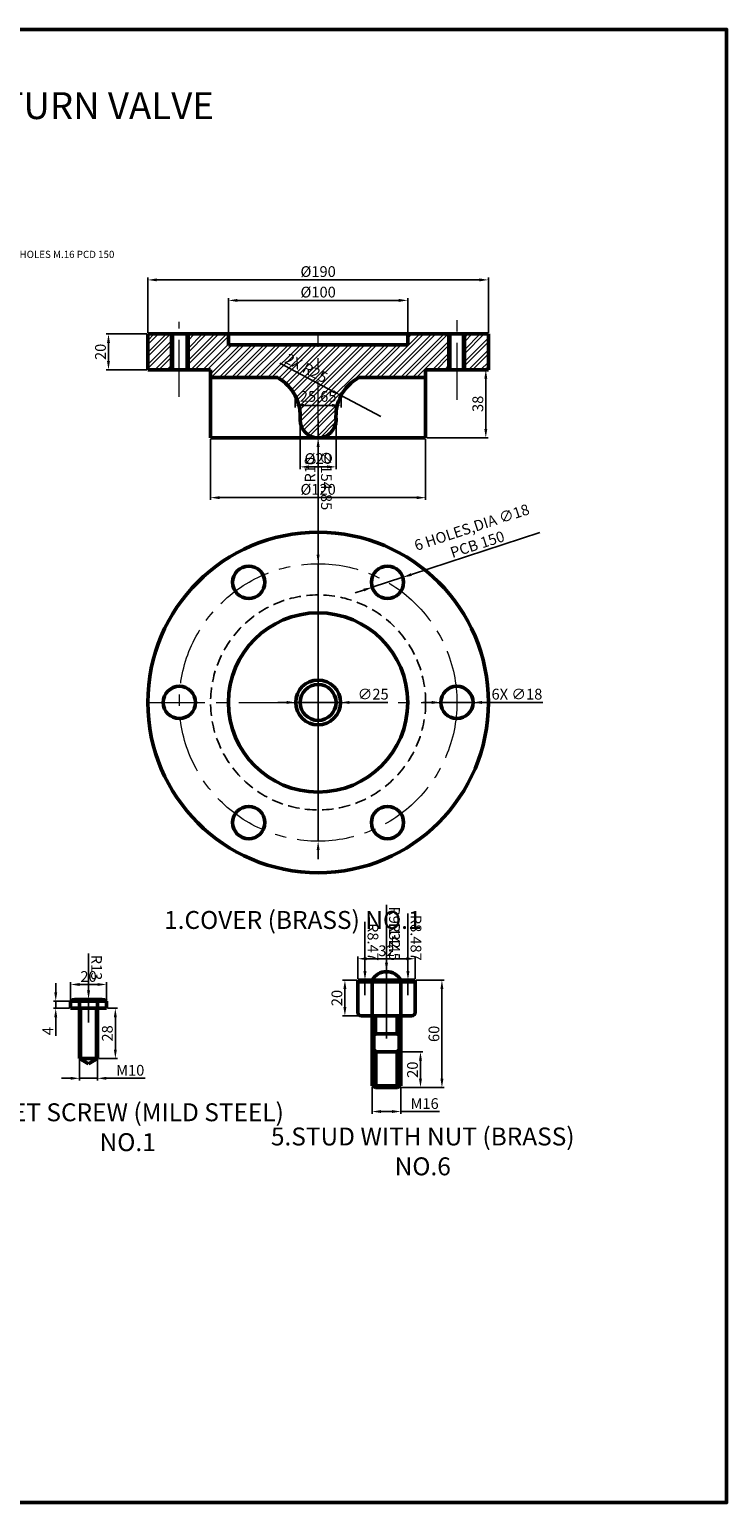
# Model space of a CAD drawing. Units: millimetres. Extents: x -907 to -46, y -312 to 510.
# Tile 3 of 3: x -434 to -46, y -312 to 510. Entities that reach past the tile are written whole.
import ezdxf
from ezdxf import colors
from ezdxf.entities.mleader import LeaderData, LeaderLine
from ezdxf.math import Vec2, Vec3

# ---------------------------------------------------------------- set-up
doc = ezdxf.new("R2010")
doc.units = ezdxf.units.MM
doc.linetypes.add('CENTER', pattern=[50.8, 31.75, -6.35, 6.35, -6.35])
doc.linetypes.add('HIDDEN', pattern=[9.525, 6.35, -3.175])
for name, color, linetype, lineweight in [('M-CNTR', 1, 'CENTER', 18), ('M-DIMS', 2, 'Continuous', 25), ('M-HATC', 8, 'Continuous', 18), ('M-HIDN', 6, 'HIDDEN', 25), ('M-OUTL', 7, 'Continuous', 50), ('M-TEXT', 3, 'Continuous', 25), ('M-TTLB', 7, 'Continuous', 50)]:
    doc.layers.add(name, color=color, linetype=linetype, lineweight=lineweight)
doc.styles.get("Standard").update_dxf_attribs({"font": 'arial.ttf'})
doc.dimstyles.new('ISO-25', dxfattribs={"dimtxt": 6, "dimasz": 5, "dimexe": 1.25, "dimexo": 0.625, "dimtad": 1, "dimtxsty": 'Standard', "dimcen": 2.5, "dimadec": 0, "dimazin": 0, "dimtfac": 1, "dimtmove": 0, "dimatfit": 3, "dimfxl": 1, "dimarcsym": 0})

# ---------------------------------------------------------------- blocks, each defined once
blk = doc.blocks.new('*D31')
at = {"layer": 'Defpoints', "color": 0, "transparency": 16777216}
for p in [(-178.39, 370.17), (-368.39, 340), (-178.39, 340)]:
    blk.add_point(p, dxfattribs=at)
at = {"layer": 'M-DIMS', "color": 0, "lineweight": -2, "transparency": 16777216}
for p, q in [((-368.39, 340.62), (-368.39, 371.42)), ((-363.39, 370.17), (-183.39, 370.17)), ((-178.39, 340.62), (-178.39, 371.42))]:
    blk.add_line(p, q, dxfattribs=at)
at = {"layer": 'M-DIMS', "color": 0, "transparency": 16777216}
for points in [[(-363.39, 371.01), (-363.39, 369.34), (-368.39, 370.17)], [(-183.39, 371.01), (-183.39, 369.34), (-178.39, 370.17)]]:
    blk.add_solid(points, dxfattribs=at)
at = {"layer": 'M-DIMS', "color": 0, "transparency": 16777216, "insert": (-273.39, 374.03), "char_height": 6, "attachment_point": 5}
blk.add_mtext('%%C190', dxfattribs=at)
blk = doc.blocks.new('*D32')
at = {"layer": 'Defpoints', "color": 0, "transparency": 16777216}
for p in [(-223.39, 358.73), (-323.39, 340), (-223.39, 340)]:
    blk.add_point(p, dxfattribs=at)
at = {"layer": 'M-DIMS', "color": 0, "lineweight": -2, "transparency": 16777216}
for p, q in [((-323.39, 340.62), (-323.39, 359.98)), ((-318.39, 358.73), (-228.39, 358.73)), ((-223.39, 340.62), (-223.39, 359.98))]:
    blk.add_line(p, q, dxfattribs=at)
at = {"layer": 'M-DIMS', "color": 0, "transparency": 16777216}
for points in [[(-318.39, 359.56), (-318.39, 357.89), (-323.39, 358.73)], [(-228.39, 359.56), (-228.39, 357.89), (-223.39, 358.73)]]:
    blk.add_solid(points, dxfattribs=at)
at = {"layer": 'M-DIMS', "color": 0, "transparency": 16777216, "insert": (-273.39, 362.58), "char_height": 6, "attachment_point": 5}
blk.add_mtext('%%C100', dxfattribs=at)
blk = doc.blocks.new('*D33')
at = {"layer": 'Defpoints', "color": 0, "transparency": 16777216}
for p in [(-368.39, 340), (-390.36, 320), (-368.39, 320)]:
    blk.add_point(p, dxfattribs=at)
at = {"layer": 'M-DIMS', "color": 0, "lineweight": -2, "transparency": 16777216}
for p, q in [((-369.02, 340), (-391.61, 340)), ((-390.36, 335), (-390.36, 325)), ((-369.02, 320), (-391.61, 320))]:
    blk.add_line(p, q, dxfattribs=at)
at = {"layer": 'M-DIMS', "color": 0, "transparency": 16777216}
for points in [[(-391.19, 335), (-389.53, 335), (-390.36, 340)], [(-391.19, 325), (-389.53, 325), (-390.36, 320)]]:
    blk.add_solid(points, dxfattribs=at)
at = {"layer": 'M-DIMS', "color": 0, "transparency": 16777216, "insert": (-394.05, 330), "char_height": 6, "attachment_point": 5, "rotation": 90}
blk.add_mtext('20', dxfattribs=at)
blk = doc.blocks.new('*D34')
at = {"layer": 'Defpoints', "color": 0, "transparency": 16777216}
for p in [(-283.39, 292), (-263.39, 292), (-263.39, 265.83)]:
    blk.add_point(p, dxfattribs=at)
at = {"layer": 'M-DIMS', "color": 0, "lineweight": -2, "transparency": 16777216}
for p, q in [((-283.39, 291.37), (-283.39, 264.58)), ((-263.39, 291.37), (-263.39, 264.58)), ((-278.39, 265.83), (-268.39, 265.83))]:
    blk.add_line(p, q, dxfattribs=at)
at = {"layer": 'M-DIMS', "color": 0, "transparency": 16777216}
for points in [[(-278.39, 266.66), (-278.39, 265), (-283.39, 265.83)], [(-268.39, 266.66), (-268.39, 265), (-263.39, 265.83)]]:
    blk.add_solid(points, dxfattribs=at)
at = {"layer": 'M-DIMS', "color": 0, "transparency": 16777216, "insert": (-273.39, 269.69), "char_height": 6, "attachment_point": 5}
blk.add_mtext('%%C20', dxfattribs=at)
blk = doc.blocks.new('*D35')
at = {"layer": 'Defpoints', "color": 0, "transparency": 16777216}
for p in [(-333.39, 282), (-213.39, 282), (-213.39, 248.65)]:
    blk.add_point(p, dxfattribs=at)
at = {"layer": 'M-DIMS', "color": 0, "lineweight": -2, "transparency": 16777216}
for p, q in [((-333.39, 281.37), (-333.39, 247.4)), ((-213.39, 281.37), (-213.39, 247.4)), ((-328.39, 248.65), (-218.39, 248.65))]:
    blk.add_line(p, q, dxfattribs=at)
at = {"layer": 'M-DIMS', "color": 0, "transparency": 16777216}
for points in [[(-328.39, 249.48), (-328.39, 247.82), (-333.39, 248.65)], [(-218.39, 249.48), (-218.39, 247.82), (-213.39, 248.65)]]:
    blk.add_solid(points, dxfattribs=at)
at = {"layer": 'M-DIMS', "color": 0, "transparency": 16777216, "insert": (-273.39, 252.51), "char_height": 6, "attachment_point": 5}
blk.add_mtext('%%C120', dxfattribs=at)
blk = doc.blocks.new('*D36')
at = {"layer": 'Defpoints', "color": 0, "transparency": 16777216}
for p in [(-286.22, 305.62), (-260.57, 305.62), (-260.57, 300.14)]:
    blk.add_point(p, dxfattribs=at)
at = {"layer": 'M-DIMS', "color": 0, "lineweight": -2, "transparency": 16777216}
for p, q in [((-286.22, 305), (-286.22, 298.89)), ((-260.57, 305), (-260.57, 298.89)), ((-281.22, 300.14), (-265.57, 300.14))]:
    blk.add_line(p, q, dxfattribs=at)
at = {"layer": 'M-DIMS', "color": 0, "transparency": 16777216}
for points in [[(-281.22, 300.97), (-281.22, 299.31), (-286.22, 300.14)], [(-265.57, 300.97), (-265.57, 299.31), (-260.57, 300.14)]]:
    blk.add_solid(points, dxfattribs=at)
at = {"layer": 'M-DIMS', "color": 0, "transparency": 16777216, "insert": (-273.39, 304.37), "char_height": 6, "attachment_point": 5}
blk.add_mtext('25,65', dxfattribs=at)
blk = doc.blocks.new('*D37')
at = {"layer": 'Defpoints', "color": 0, "transparency": 16777216}
for p in [(-213.39, 320), (-213.39, 282), (-179.83, 282)]:
    blk.add_point(p, dxfattribs=at)
at = {"layer": 'M-DIMS', "color": 0, "lineweight": -2, "transparency": 16777216}
for p, q in [((-212.77, 320), (-178.58, 320)), ((-179.83, 315), (-179.83, 287)), ((-212.77, 282), (-178.58, 282))]:
    blk.add_line(p, q, dxfattribs=at)
at = {"layer": 'M-DIMS', "color": 0, "transparency": 16777216}
for points in [[(-180.66, 315), (-179, 315), (-179.83, 320)], [(-180.66, 287), (-179, 287), (-179.83, 282)]]:
    blk.add_solid(points, dxfattribs=at)
at = {"layer": 'M-DIMS', "color": 0, "transparency": 16777216, "insert": (-183.52, 301), "char_height": 6, "attachment_point": 5, "rotation": 90}
blk.add_mtext('38', dxfattribs=at)
blk = doc.blocks.new('*D38')
at = {"layer": 'Defpoints', "color": 0, "transparency": 16777216}
for p in [(-243.24, 198.61), (-226.12, 204.19)]:
    blk.add_point(p, dxfattribs=at)
at = {"layer": 'M-DIMS', "color": 0, "lineweight": -2, "transparency": 16777216}
for p, q in [((-149.63, 229.11), (-221.37, 205.74)), ((-243.24, 198.61), (-226.12, 204.19)), ((-247.99, 197.07), (-252.75, 195.52))]:
    blk.add_line(p, q, dxfattribs=at)
at = {"layer": 'M-DIMS', "color": 0, "transparency": 16777216}
for points in [[(-221.63, 206.53), (-221.11, 204.95), (-226.12, 204.19)], [(-248.25, 197.86), (-247.73, 196.27), (-243.24, 198.61)]]:
    blk.add_solid(points, dxfattribs=at)
at = {"layer": 'M-DIMS', "color": 0, "transparency": 16777216, "insert": (-185.86, 226.6), "char_height": 6, "attachment_point": 5, "rotation": 18.0433}
blk.add_mtext('6 HOLES,DIA ∅18\\PPCB 150', dxfattribs=at)
blk = doc.blocks.new('*D49')
at = {"layer": 'Defpoints', "color": 0, "transparency": 16777216}
for p in [(-406.48, -64.34), (-396.48, -64.34), (-396.48, -75.39)]:
    blk.add_point(p, dxfattribs=at)
at = {"layer": 'M-DIMS', "color": 0, "lineweight": -2, "transparency": 16777216}
for p, q in [((-406.48, -64.97), (-406.48, -76.64)), ((-396.48, -64.97), (-396.48, -76.64)), ((-411.48, -75.39), (-416.48, -75.39)), ((-406.48, -75.39), (-396.48, -75.39)), ((-391.48, -75.39), (-369.95, -75.39))]:
    blk.add_line(p, q, dxfattribs=at)
at = {"layer": 'M-DIMS', "color": 0, "transparency": 16777216}
for points in [[(-411.48, -74.56), (-411.48, -76.23), (-406.48, -75.39)], [(-391.48, -74.56), (-391.48, -76.23), (-396.48, -75.39)]]:
    blk.add_solid(points, dxfattribs=at)
at = {"layer": 'M-DIMS', "color": 0, "transparency": 16777216, "insert": (-378.22, -71.7), "char_height": 6, "attachment_point": 5}
blk.add_mtext('M10', dxfattribs=at)
blk = doc.blocks.new('*D50')
at = {"layer": 'Defpoints', "color": 0, "transparency": 16777216}
for p in [(-219.25, -20.59), (-235.25, -80.59), (-204.32, -80.59)]:
    blk.add_point(p, dxfattribs=at)
at = {"layer": 'M-DIMS', "color": 0, "lineweight": -2, "transparency": 16777216}
for p, q in [((-218.63, -20.59), (-203.07, -20.59)), ((-204.32, -25.59), (-204.32, -75.59)), ((-234.63, -80.59), (-203.07, -80.59))]:
    blk.add_line(p, q, dxfattribs=at)
at = {"layer": 'M-DIMS', "color": 0, "transparency": 16777216}
for points in [[(-205.15, -25.59), (-203.48, -25.59), (-204.32, -20.59)], [(-205.15, -75.59), (-203.48, -75.59), (-204.32, -80.59)]]:
    blk.add_solid(points, dxfattribs=at)
at = {"layer": 'M-DIMS', "color": 0, "transparency": 16777216, "insert": (-208, -50.59), "char_height": 6, "attachment_point": 5, "rotation": 90}
blk.add_mtext('60', dxfattribs=at)
blk = doc.blocks.new('*D51')
at = {"layer": 'Defpoints', "color": 0, "transparency": 16777216}
for p in [(-235.25, -60.59), (-235.25, -80.59), (-216.29, -80.59)]:
    blk.add_point(p, dxfattribs=at)
at = {"layer": 'M-DIMS', "color": 0, "lineweight": -2, "transparency": 16777216}
for p, q in [((-234.63, -60.59), (-215.04, -60.59)), ((-216.29, -65.59), (-216.29, -75.59)), ((-234.63, -80.59), (-215.04, -80.59))]:
    blk.add_line(p, q, dxfattribs=at)
at = {"layer": 'M-DIMS', "color": 0, "transparency": 16777216}
for points in [[(-217.12, -65.59), (-215.45, -65.59), (-216.29, -60.59)], [(-217.12, -75.59), (-215.45, -75.59), (-216.29, -80.59)]]:
    blk.add_solid(points, dxfattribs=at)
at = {"layer": 'M-DIMS', "color": 0, "transparency": 16777216, "insert": (-219.97, -70.59), "char_height": 6, "attachment_point": 5, "rotation": 90}
blk.add_mtext('20', dxfattribs=at)
blk = doc.blocks.new('*D52')
at = {"layer": 'Defpoints', "color": 0, "transparency": 16777216}
for p in [(-243.25, -79.59), (-227.25, -79.59), (-227.25, -93.95)]:
    blk.add_point(p, dxfattribs=at)
at = {"layer": 'M-DIMS', "color": 0, "lineweight": -2, "transparency": 16777216}
for p, q in [((-243.25, -80.22), (-243.25, -95.2)), ((-227.25, -80.22), (-227.25, -95.2)), ((-238.25, -93.95), (-232.25, -93.95)), ((-227.25, -93.95), (-205.7, -93.95))]:
    blk.add_line(p, q, dxfattribs=at)
at = {"layer": 'M-DIMS', "color": 0, "transparency": 16777216}
for points in [[(-238.25, -93.11), (-238.25, -94.78), (-243.25, -93.95)], [(-232.25, -93.11), (-232.25, -94.78), (-227.25, -93.95)]]:
    blk.add_solid(points, dxfattribs=at)
at = {"layer": 'M-DIMS', "color": 0, "transparency": 16777216, "insert": (-213.98, -90.26), "char_height": 6, "attachment_point": 5}
blk.add_mtext('M16', dxfattribs=at)
blk = doc.blocks.new('*D53')
at = {"layer": 'Defpoints', "color": 0, "transparency": 16777216}
for p in [(-391.48, -36.34), (-396.48, -64.34), (-386.53, -64.34)]:
    blk.add_point(p, dxfattribs=at)
at = {"layer": 'M-DIMS', "color": 0, "lineweight": -2, "transparency": 16777216}
for p, q in [((-390.86, -36.34), (-385.28, -36.34)), ((-386.53, -41.34), (-386.53, -59.34)), ((-395.86, -64.34), (-385.28, -64.34))]:
    blk.add_line(p, q, dxfattribs=at)
at = {"layer": 'M-DIMS', "color": 0, "transparency": 16777216}
for points in [[(-387.36, -41.34), (-385.7, -41.34), (-386.53, -36.34)], [(-387.36, -59.34), (-385.7, -59.34), (-386.53, -64.34)]]:
    blk.add_solid(points, dxfattribs=at)
at = {"layer": 'M-DIMS', "color": 0, "transparency": 16777216, "insert": (-390.22, -50.34), "char_height": 6, "attachment_point": 5, "rotation": 90}
blk.add_mtext('28', dxfattribs=at)
blk = doc.blocks.new('HOLE-D18')
blk.add_circle((9, 9), 9)
blk = doc.blocks.new('*D57')
at = {"layer": 'Defpoints', "color": 0, "transparency": 16777216}
for p in [(-391.48, -23.04), (-411.48, -36.34), (-391.48, -36.34)]:
    blk.add_point(p, dxfattribs=at)
at = {"layer": 'M-DIMS', "color": 0, "lineweight": -2, "transparency": 16777216}
for p, q in [((-411.48, -35.72), (-411.48, -21.79)), ((-406.48, -23.04), (-396.48, -23.04)), ((-391.48, -35.72), (-391.48, -21.79))]:
    blk.add_line(p, q, dxfattribs=at)
at = {"layer": 'M-DIMS', "color": 0, "transparency": 16777216}
for points in [[(-406.48, -22.21), (-406.48, -23.87), (-411.48, -23.04)], [(-396.48, -22.21), (-396.48, -23.87), (-391.48, -23.04)]]:
    blk.add_solid(points, dxfattribs=at)
at = {"layer": 'M-DIMS', "color": 0, "transparency": 16777216, "insert": (-401.48, -19.35), "char_height": 6, "attachment_point": 5}
blk.add_mtext('20', dxfattribs=at)
blk = doc.blocks.new('*D58')
at = {"layer": 'Defpoints', "color": 0, "transparency": 16777216}
for p in [(-411.48, -32.34), (-419.78, -36.34), (-411.48, -36.34)]:
    blk.add_point(p, dxfattribs=at)
at = {"layer": 'M-DIMS', "color": 0, "lineweight": -2, "transparency": 16777216}
for p, q in [((-419.78, -27.34), (-419.78, -22.34)), ((-412.11, -32.34), (-421.03, -32.34)), ((-419.78, -32.34), (-419.78, -36.34)), ((-412.11, -36.34), (-421.03, -36.34)), ((-419.78, -41.34), (-419.78, -51.74))]:
    blk.add_line(p, q, dxfattribs=at)
at = {"layer": 'M-DIMS', "color": 0, "transparency": 16777216}
for points in [[(-420.62, -27.34), (-418.95, -27.34), (-419.78, -32.34)], [(-420.62, -41.34), (-418.95, -41.34), (-419.78, -36.34)]]:
    blk.add_solid(points, dxfattribs=at)
at = {"layer": 'M-DIMS', "color": 0, "transparency": 16777216, "insert": (-423.41, -49.04), "char_height": 6, "attachment_point": 5, "rotation": 90}
blk.add_mtext('4', dxfattribs=at)
blk = doc.blocks.new('*D59')
at = {"layer": 'Defpoints', "color": 0, "transparency": 16777216}
for p in [(-219.25, -8.68), (-251.25, -20.59), (-219.25, -20.59)]:
    blk.add_point(p, dxfattribs=at)
at = {"layer": 'M-DIMS', "color": 0, "lineweight": -2, "transparency": 16777216}
for p, q in [((-251.25, -19.97), (-251.25, -7.43)), ((-219.25, -19.97), (-219.25, -7.43)), ((-246.25, -8.68), (-224.25, -8.68))]:
    blk.add_line(p, q, dxfattribs=at)
at = {"layer": 'M-DIMS', "color": 0, "transparency": 16777216}
for points in [[(-246.25, -7.85), (-246.25, -9.51), (-251.25, -8.68)], [(-224.25, -7.85), (-224.25, -9.51), (-219.25, -8.68)]]:
    blk.add_solid(points, dxfattribs=at)
at = {"layer": 'M-DIMS', "color": 0, "transparency": 16777216, "insert": (-235.25, -4.99), "char_height": 6, "attachment_point": 5}
blk.add_mtext('32', dxfattribs=at)
blk = doc.blocks.new('*D60')
at = {"layer": 'Defpoints', "color": 0, "transparency": 16777216}
for p in [(-251.25, -20.59), (-258.45, -40.59), (-249.25, -40.59)]:
    blk.add_point(p, dxfattribs=at)
at = {"layer": 'M-DIMS', "color": 0, "lineweight": -2, "transparency": 16777216}
for p, q in [((-251.88, -20.59), (-259.7, -20.59)), ((-258.45, -25.59), (-258.45, -35.59)), ((-249.88, -40.59), (-259.7, -40.59))]:
    blk.add_line(p, q, dxfattribs=at)
at = {"layer": 'M-DIMS', "color": 0, "transparency": 16777216}
for points in [[(-259.29, -25.59), (-257.62, -25.59), (-258.45, -20.59)], [(-259.29, -35.59), (-257.62, -35.59), (-258.45, -40.59)]]:
    blk.add_solid(points, dxfattribs=at)
at = {"layer": 'M-DIMS', "color": 0, "transparency": 16777216, "insert": (-262.14, -30.59), "char_height": 6, "attachment_point": 5, "rotation": 90}
blk.add_mtext('20', dxfattribs=at)
blk = doc.blocks.new('*D64')
at = {"layer": 'Defpoints', "color": 0, "transparency": 16777216}
for p in [(-260.57, 305.62), (-238.47, 293.93)]:
    blk.add_point(p, dxfattribs=at)
at = {"layer": 'M-DIMS', "color": 0, "lineweight": -2, "transparency": 16777216}
for p, q in [((-294.71, 323.68), (-264.99, 307.96)), ((-238.47, 293.93), (-260.57, 305.62))]:
    blk.add_line(p, q, dxfattribs=at)
at = {"layer": 'M-DIMS', "color": 0, "transparency": 16777216}
blk.add_solid([(-264.6, 308.7), (-265.38, 307.22), (-260.57, 305.62)], dxfattribs=at)
at = {"layer": 'M-DIMS', "color": 0, "transparency": 16777216, "insert": (-280.33, 320.25), "char_height": 6, "attachment_point": 5, "rotation": 332.11935}
blk.add_mtext('2X R25', dxfattribs=at)
blk = doc.blocks.new('*D65')
at = {"layer": 'Defpoints', "color": 0, "transparency": 16777216}
for p in [(-273.39, 292), (-273.39, 282)]:
    blk.add_point(p, dxfattribs=at)
at = {"layer": 'M-DIMS', "color": 0, "lineweight": -2, "transparency": 16777216}
for p, q in [((-273.39, 292), (-273.39, 282)), ((-273.39, 256.43), (-273.39, 277))]:
    blk.add_line(p, q, dxfattribs=at)
at = {"layer": 'M-DIMS', "color": 0, "transparency": 16777216}
blk.add_solid([(-274.23, 277), (-272.56, 277), (-273.39, 282)], dxfattribs=at)
at = {"layer": 'M-DIMS', "color": 0, "transparency": 16777216, "insert": (-277.08, 264.21), "char_height": 6, "attachment_point": 5, "rotation": 89.99849}
blk.add_mtext('R10', dxfattribs=at)
blk = doc.blocks.new('*D66')
at = {"layer": 'Defpoints', "color": 0, "transparency": 16777216}
for p in [(-204.97, 134.35), (-186.97, 134.35)]:
    blk.add_point(p, dxfattribs=at)
at = {"layer": 'M-DIMS', "color": 0, "lineweight": -2, "transparency": 16777216}
for p, q in [((-209.97, 134.35), (-214.97, 134.35)), ((-204.97, 134.35), (-186.97, 134.35)), ((-147.98, 134.35), (-181.97, 134.35))]:
    blk.add_line(p, q, dxfattribs=at)
at = {"layer": 'M-DIMS', "color": 0, "transparency": 16777216}
for points in [[(-209.97, 135.19), (-209.97, 133.52), (-204.97, 134.35)], [(-181.97, 135.19), (-181.97, 133.52), (-186.97, 134.35)]]:
    blk.add_solid(points, dxfattribs=at)
at = {"layer": 'M-DIMS', "color": 0, "transparency": 16777216, "insert": (-162.47, 138.21), "char_height": 6, "attachment_point": 5, "rotation": 359.99799}
blk.add_mtext('6X ∅18', dxfattribs=at)
blk = doc.blocks.new('*D67')
at = {"layer": 'Defpoints', "color": 0, "transparency": 16777216}
for p in [(-273.39, 211.77), (-273.39, 56.93)]:
    blk.add_point(p, dxfattribs=at)
at = {"layer": 'M-DIMS', "color": 0, "lineweight": -2, "transparency": 16777216}
for p, q in [((-273.39, 274.59), (-273.39, 216.77)), ((-273.39, 56.93), (-273.39, 211.77)), ((-273.39, 51.93), (-273.39, 46.93))]:
    blk.add_line(p, q, dxfattribs=at)
at = {"layer": 'M-DIMS', "color": 0, "transparency": 16777216}
for points in [[(-272.56, 216.77), (-274.23, 216.77), (-273.39, 211.77)], [(-272.56, 51.93), (-274.23, 51.93), (-273.39, 56.93)]]:
    blk.add_solid(points, dxfattribs=at)
at = {"layer": 'M-DIMS', "color": 0, "transparency": 16777216, "insert": (-269.54, 258.23), "char_height": 6, "attachment_point": 5, "rotation": 270.00019}
blk.add_mtext('∅154.85', dxfattribs=at)
blk = doc.blocks.new('*D68')
at = {"layer": 'Defpoints', "color": 0, "transparency": 16777216}
for p in [(-285.89, 134.35), (-260.89, 134.35)]:
    blk.add_point(p, dxfattribs=at)
at = {"layer": 'M-DIMS', "color": 0, "lineweight": -2, "transparency": 16777216}
for p, q in [((-290.89, 134.35), (-295.89, 134.35)), ((-285.89, 134.35), (-260.89, 134.35)), ((-234.47, 134.35), (-255.89, 134.35))]:
    blk.add_line(p, q, dxfattribs=at)
at = {"layer": 'M-DIMS', "color": 0, "transparency": 16777216}
for points in [[(-290.89, 135.19), (-290.89, 133.52), (-285.89, 134.35)], [(-255.89, 135.19), (-255.89, 133.52), (-260.89, 134.35)]]:
    blk.add_solid(points, dxfattribs=at)
at = {"layer": 'M-DIMS', "color": 0, "transparency": 16777216, "insert": (-242.68, 138.21), "char_height": 6, "attachment_point": 5, "rotation": 359.99857}
blk.add_mtext('∅25', dxfattribs=at)
blk = doc.blocks.new('*D69')
at = {"layer": 'Defpoints', "color": 0, "transparency": 16777216}
for p in [(-401.48, -31.34), (-401.48, -44.34)]:
    blk.add_point(p, dxfattribs=at)
at = {"layer": 'M-DIMS', "color": 0, "lineweight": -2, "transparency": 16777216}
for p, q in [((-401.48, -5.75), (-401.48, -26.34)), ((-401.48, -44.34), (-401.48, -31.34))]:
    blk.add_line(p, q, dxfattribs=at)
at = {"layer": 'M-DIMS', "color": 0, "transparency": 16777216}
blk.add_solid([(-400.65, -26.34), (-402.32, -26.34), (-401.48, -31.34)], dxfattribs=at)
at = {"layer": 'M-DIMS', "color": 0, "transparency": 16777216, "insert": (-397.79, -13.55), "char_height": 6, "attachment_point": 5, "rotation": 270.00195}
blk.add_mtext('R13', dxfattribs=at)
blk = doc.blocks.new('*D70')
at = {"layer": 'Defpoints', "color": 0, "transparency": 16777216}
for p in [(-235.25, -20.59), (-235.25, -53.09)]:
    blk.add_point(p, dxfattribs=at)
at = {"layer": 'M-DIMS', "color": 0, "lineweight": -2, "transparency": 16777216}
for p, q in [((-235.25, 12.03), (-235.25, -15.59)), ((-235.25, -53.09), (-235.25, -20.59))]:
    blk.add_line(p, q, dxfattribs=at)
at = {"layer": 'M-DIMS', "color": 0, "transparency": 16777216}
blk.add_solid([(-234.42, -15.59), (-236.09, -15.59), (-235.25, -20.59)], dxfattribs=at)
at = {"layer": 'M-DIMS', "color": 0, "transparency": 16777216, "insert": (-231.56, 0.72), "char_height": 6, "attachment_point": 5, "rotation": 270.00062}
blk.add_mtext('R32.5', dxfattribs=at)
blk = doc.blocks.new('*D71')
at = {"layer": 'Defpoints', "color": 0, "transparency": 16777216}
for p in [(-235.25, -15.88), (-235.25, -25.02)]:
    blk.add_point(p, dxfattribs=at)
at = {"layer": 'M-DIMS', "color": 0, "lineweight": -2, "transparency": 16777216}
for p, q in [((-235.25, 21.34), (-235.25, -10.88)), ((-235.25, -25.02), (-235.25, -15.88))]:
    blk.add_line(p, q, dxfattribs=at)
at = {"layer": 'M-DIMS', "color": 0, "transparency": 16777216}
blk.add_solid([(-234.42, -10.88), (-236.09, -10.88), (-235.25, -15.88)], dxfattribs=at)
at = {"layer": 'M-DIMS', "color": 0, "transparency": 16777216, "insert": (-231.57, 7.73), "char_height": 6, "attachment_point": 5, "rotation": 270.0022}
blk.add_mtext('R9.144', dxfattribs=at)
blk = doc.blocks.new('*D72')
at = {"layer": 'Defpoints', "color": 0, "transparency": 16777216}
for p in [(-247.25, -20.59), (-247.25, -29.06)]:
    blk.add_point(p, dxfattribs=at)
at = {"layer": 'M-DIMS', "color": 0, "lineweight": -2, "transparency": 16777216}
for p, q in [((-247.25, 11.99), (-247.25, -15.59)), ((-247.25, -29.06), (-247.25, -20.59))]:
    blk.add_line(p, q, dxfattribs=at)
at = {"layer": 'M-DIMS', "color": 0, "transparency": 16777216}
blk.add_solid([(-246.42, -15.59), (-248.09, -15.59), (-247.25, -20.59)], dxfattribs=at)
at = {"layer": 'M-DIMS', "color": 0, "transparency": 16777216, "insert": (-243.57, 0.7), "char_height": 6, "attachment_point": 5, "rotation": 270.00237}
blk.add_mtext('R8.47', dxfattribs=at)
blk = doc.blocks.new('*D73')
at = {"layer": 'Defpoints', "color": 0, "transparency": 16777216}
for p in [(-223.25, -20.59), (-223.25, -29.08)]:
    blk.add_point(p, dxfattribs=at)
at = {"layer": 'M-DIMS', "color": 0, "lineweight": -2, "transparency": 16777216}
for p, q in [((-223.25, 16.65), (-223.25, -15.59)), ((-223.25, -29.08), (-223.25, -20.59))]:
    blk.add_line(p, q, dxfattribs=at)
at = {"layer": 'M-DIMS', "color": 0, "transparency": 16777216}
blk.add_solid([(-222.42, -15.59), (-224.09, -15.59), (-223.25, -20.59)], dxfattribs=at)
at = {"layer": 'M-DIMS', "color": 0, "transparency": 16777216, "insert": (-219.57, 3.03), "char_height": 6, "attachment_point": 5, "rotation": 270.00237}
blk.add_mtext('R8.487', dxfattribs=at)

msp = doc.modelspace()

# ---------------------------------------------------------------- hatches: boundary and pattern name
at = {"layer": 'M-HATC'}
h = msp.add_hatch(dxfattribs=at)
h.set_pattern_fill('ANSI32', color=256, scale=0.5)
h.set_pattern_definition([(45, (-1262.664, -275.01), (-3.367596, 3.367596), []), (45, (-1260.419, -275.01), (-3.367596, 3.367596), [])])
h.paths.add_polyline_path([(-273.3927, 333.9967), (-323.3927, 333.9967), (-323.3927, 339.9967), (-345.8927, 339.9967), (-345.8927, 319.9967), (-333.3927, 319.9967), (-333.3927, 315.6248), (-295.8927, 315.6248, -0.28975103), (-283.3927, 291.9967, 0.41421356), (-273.3927, 281.9967)])
h.paths.add_polyline_path([(-200.3996, 339.9967), (-223.3927, 339.9967), (-223.3927, 333.9967), (-273.3927, 333.9967), (-273.3927, 281.9967, 0.41421356), (-263.3927, 291.9967, -0.28975103), (-250.8927, 315.6248), (-213.3927, 315.6248), (-213.3927, 319.9967), (-200.3996, 319.9967)])
h.paths.add_polyline_path([(-355.2229, 339.9967), (-368.3927, 339.9967), (-368.3927, 319.9967), (-355.2229, 319.9967)])
h.paths.add_polyline_path([(-178.3927, 339.9967), (-191.7391, 339.9967), (-191.7391, 319.9967), (-178.3927, 319.9967)])

# ---------------------------------------------------------------- linework, layer by layer
at = {"layer": 'M-CNTR'}
for p, q in [((-350.8927, 304.8881), (-350.8927, 346.7716)), ((-195.8927, 303.2568), (-195.8927, 349.0138)), ((-273.3927, 281.9967), (-273.3927, 339.9967)), ((-273.3927, 254.0317), (-273.3927, 54.4385)), ((-368.3927, 134.3523), (-178.3927, 134.3523))]:
    msp.add_line(p, q, dxfattribs=at)
msp.add_circle((-273.3927, 134.3523), 77.4225, dxfattribs=at)
at = {"layer": 'M-HIDN'}
msp.add_circle((-273.3927, 134.3523), 60, dxfattribs=at)
at = {"layer": 'M-OUTL'}
for p, q in [((-368.3927, 339.9967), (-178.3927, 339.9967)), ((-368.3927, 319.9967), (-368.3927, 339.9967)), ((-355.2229, 319.9967), (-355.2229, 339.9967)), ((-354.7229, 319.9967), (-354.7229, 339.9967)), ((-346.3927, 319.9967), (-346.3927, 339.9967)), ((-345.8927, 319.9967), (-345.8927, 339.9967)), ((-323.3927, 333.9967), (-323.3927, 339.9967)), ((-223.3927, 333.9967), (-223.3927, 339.9967)), ((-200.3996, 319.9967), (-200.3996, 339.9967)), ((-199.8996, 319.9967), (-199.8996, 339.9967)), ((-192.2391, 319.9967), (-192.2391, 339.9967)), ((-191.7391, 319.9967), (-191.7391, 339.9967)), ((-178.3927, 339.9967), (-178.3927, 319.9967)), ((-223.3927, 333.9967), (-323.3927, 333.9967)), ((-368.3927, 319.9967), (-333.3927, 319.9967)), ((-333.3927, 319.9967), (-333.3927, 281.9967)), ((-295.8927, 315.6248), (-333.3927, 315.6248)), ((-213.3927, 315.6248), (-250.8927, 315.6248)), ((-213.3927, 281.9967), (-213.3927, 319.9967)), ((-213.3927, 319.9967), (-178.3927, 319.9967)), ((-333.3927, 281.9967), (-213.3927, 281.9967)), ((-251.2526, -20.594), (-219.2526, -20.594)), ((-251.2526, -38.594), (-251.2526, -20.594)), ((-251.2526, -21.594), (-219.2526, -21.594)), ((-243.2526, -20.594), (-243.2526, -79.594)), ((-227.2526, -79.594), (-227.2526, -20.594)), ((-219.2526, -20.594), (-219.2526, -38.594)), ((-411.4836, -32.3418), (-411.4836, -36.3418)), ((-391.4836, -32.3418), (-411.4836, -32.3418)), ((-393.9325, -31.3418), (-409.0902, -31.3418)), ((-406.4836, -31.3418), (-406.4836, -64.3418)), ((-396.4836, -64.3418), (-396.4836, -31.3418)), ((-391.4836, -36.3418), (-391.4836, -32.3418)), ((-411.4836, -36.3418), (-406.4836, -36.3418)), ((-396.4836, -36.3418), (-406.4836, -36.3418)), ((-405.9836, -36.3418), (-405.9836, -64.3418)), ((-396.9836, -64.3418), (-396.9836, -36.3418)), ((-396.4836, -36.3418), (-391.4836, -36.3418)), ((-221.2526, -40.594), (-249.2526, -40.594)), ((-241.4111, -50.5025), (-241.4111, -40.594)), ((-229.2526, -50.594), (-229.2526, -40.594)), ((-242.2526, -51.594), (-241.2526, -50.594)), ((-242.2526, -51.594), (-242.2526, -59.594)), ((-241.2526, -50.594), (-229.2526, -50.594)), ((-229.2526, -50.594), (-228.2526, -51.594)), ((-228.2526, -59.594), (-228.2526, -51.594)), ((-406.4836, -64.3418), (-396.4836, -64.3418)), ((-406.4836, -64.3418), (-401.4836, -67.2285)), ((-396.4836, -64.3418), (-401.4836, -67.2285)), ((-242.2526, -59.594), (-241.2526, -60.594)), ((-241.2526, -60.594), (-229.2526, -60.594)), ((-241.2526, -60.594), (-241.2526, -80.594)), ((-228.2526, -59.594), (-229.2526, -60.594)), ((-229.2526, -60.594), (-229.2526, -80.594)), ((-243.2526, -79.594), (-227.2526, -79.594)), ((-243.2526, -79.594), (-241.2526, -80.594)), ((-241.2526, -80.594), (-229.2526, -80.594)), ((-227.2526, -79.594), (-229.2526, -80.594))]:
    msp.add_line(p, q, dxfattribs=at)
for radius in [95, 50, 12.5, 10]:
    msp.add_circle((-273.3927, 134.3523), radius, dxfattribs=at)
for centre, radius, start, end in [((-308.3178, 293.9311), 25, 355.5621585, 60.1981576), ((-238.4677, 293.9311), 25, 119.8018424, 184.4378415), ((-273.3927, 291.9967), 10, 180, 0), ((-235.2526, -25.0234), 9.1444, 28.9723486, 151.0276514), ((-247.2526, -29.0597), 8.4697, 61.8181922, 118.1818078), ((-235.2526, -53.094), 32.5, 75.7499673, 104.2500327), ((-223.2526, -29.079), 8.4868, 61.8798079, 118.1201921), ((-408.9836, -34.9611), 3.6209, 46.3350868, 133.6649132), ((-401.4836, -44.3418), 13, 67.3801351, 112.6198649), ((-393.9836, -34.9655), 3.6241, 46.3829852, 133.6170148), ((-249.2526, -38.594), 2, 180, 270), ((-221.2526, -38.594), 2, 270, 0)]:
    msp.add_arc(centre, radius, start, end, dxfattribs=at)
at = {"layer": 'M-TTLB'}
msp.add_lwpolyline([(-906.9397, 509.9283), (-45.5255, 509.9283), (-45.5255, -312.1438), (-906.9397, -312.1438)], close=True, dxfattribs=at)

# ---------------------------------------------------------------- block references
at = {"layer": 'M-OUTL'}
for p in [(-321.1038, 192.4019), (-243.6813, 192.4019), (-359.8151, 125.352), (-204.97, 125.352), (-321.1038, 58.3021), (-243.6813, 58.3021)]:
    msp.add_blockref('HOLE-D18', p, dxfattribs=at)

# ---------------------------------------------------------------- texts
at = {"layer": 'M-TEXT', "attachment_point": 1}
for s, width, insert, char_height in [('\\pxqc;NON RETURN VALVE', 433.762066, (-644.8993, 474.9186), 15), ('1.COVER (BRASS) NO.1 ', 178.714279, (-359.3224, 17.9694), 10), ('\\pxqc;6. SET SCREW (MILD STEEL) NO.1 ', 178.714279, (-469.0108, -89.3586), 10), ('\\pxqc;5.STUD WITH NUT (BRASS) NO.6', 178.714279, (-304.3745, -102.8561), 10)]:
    msp.add_mtext_dynamic_manual_height_columns(s, width=width, gutter_width=12.5, heights=[0], dxfattribs=dict(at, insert=insert, char_height=char_height))

# ---------------------------------------------------------------- dimensions: what is measured, and where the dimension line sits
at = {"layer": 'M-DIMS'}
for base, p1, p2, picture, middle in [((-178.3927, 370.1726), (-368.3927, 339.9967), (-178.3927, 339.9967), '*D31', (-273.3927, 370.1726)), ((-263.3927, 265.83), (-283.3927, 291.9967), (-263.3927, 291.9967), '*D34', (-273.3927, 265.83)), ((-213.3927, 248.6495), (-333.3927, 281.9967), (-213.3927, 281.9967), '*D35', (-273.3927, 248.6495))]:
    dim = msp.add_linear_dim(base=base, p1=p1, p2=p2, text='%%C<>', dimstyle='ISO-25', override={"dimclrd": 0, "dimclre": 0, "dimclrt": 0}, dxfattribs=at)
    dim.commit()
    dim.dimension.update_dxf_attribs({"geometry": picture, "text_midpoint": middle, "dimtype": 160})
for base, p1, p2, text, picture, middle in [((-223.3927, 358.7256), (-323.3927, 339.9967), (-223.3927, 339.9967), '%%C<>', '*D32', (-273.3927, 362.5818)), ((-396.4836, -75.3929), (-406.4836, -64.3418), (-396.4836, -64.3418), 'M<>', '*D49', (-378.2174, -71.7045)), ((-227.2526, -93.9455), (-243.2526, -79.594), (-227.2526, -79.594), 'M<>', '*D52', (-213.9783, -90.2571))]:
    dim = msp.add_linear_dim(base=base, p1=p1, p2=p2, text=text, dimstyle='ISO-25', override={"dimclrd": 0, "dimclre": 0, "dimclrt": 0}, dxfattribs=at)
    dim.commit()
    dim.dimension.update_dxf_attribs({"geometry": picture, "text_midpoint": middle})
for base, p1, p2, override, picture, middle in [((-390.3598, 319.9967), (-368.3927, 339.9967), (-368.3927, 319.9967), {"dimclrd": 0, "dimclre": 0, "dimclrt": 0}, '*D33', (-394.0482, 329.9967)), ((-179.8311, 281.9967), (-213.3927, 319.9967), (-213.3927, 281.9967), {"dimclrd": 0, "dimclre": 0, "dimclrt": 0}, '*D37', (-183.5216, 300.9967)), ((-419.7836, -36.3418), (-411.4836, -32.3418), (-411.4836, -36.3418), {"dimdec": 0, "dimlfac": 1, "dimrnd": 0, "dimzin": 0, "dimdsep": 46, "dimlunit": 2}, '*D58', (-423.4086, -49.0418)), ((-258.4526, -40.594), (-251.2526, -20.594), (-249.2526, -40.594), {"dimdec": 0, "dimlfac": 1, "dimrnd": 0, "dimzin": 0, "dimdsep": 46, "dimlunit": 2}, '*D60', (-262.1411, -30.594)), ((-204.3163, -80.594), (-219.2526, -20.594), (-235.2526, -80.594), {"dimclrd": 0, "dimclre": 0, "dimclrt": 0}, '*D50', (-208.0047, -50.594)), ((-386.5309, -64.3418), (-391.4836, -36.3418), (-396.4836, -64.3418), {"dimclrd": 0, "dimclre": 0, "dimclrt": 0}, '*D53', (-390.2194, -50.3418)), ((-216.2855, -80.594), (-235.2526, -60.594), (-235.2526, -80.594), {"dimclrd": 0, "dimclre": 0, "dimclrt": 0}, '*D51', (-219.9739, -70.594))]:
    dim = msp.add_linear_dim(base=base, p1=p1, p2=p2, angle=90, dimstyle='ISO-25', override=override, dxfattribs=at)
    dim.commit()
    dim.dimension.update_dxf_attribs({"geometry": picture, "text_midpoint": middle})
dim = msp.add_radius_dim(center=(-238.4677, 293.9311), mpoint=(-260.5658, 305.6219), text='2X <>', dimstyle='ISO-25', override={"dimdec": 0, "dimlfac": 1, "dimrnd": 0, "dimzin": 0, "dimdsep": 46, "dimlunit": 2}, dxfattribs=at)
dim.commit()
dim.dimension.update_dxf_attribs({"geometry": '*D64', "text_midpoint": (-280.332, 320.2518)})
for base, p1, p2, override, picture, middle in [((-260.5659, 300.1395), (-286.2196, 305.6217), (-260.5659, 305.6217), {"dimclrd": 0, "dimclre": 0, "dimclrt": 0}, '*D36', (-273.3927, 304.3703)), ((-219.2526, -8.679), (-251.2526, -20.594), (-219.2526, -20.594), {"dimdec": 0, "dimlfac": 1, "dimrnd": 0, "dimzin": 0, "dimdsep": 46, "dimlunit": 2}, '*D59', (-235.2526, -4.9886)), ((-391.4836, -23.0402), (-411.4836, -36.3418), (-391.4836, -36.3418), {"dimdec": 0, "dimlfac": 1, "dimrnd": 0, "dimzin": 0, "dimdsep": 46, "dimlunit": 2}, '*D57', (-401.4836, -19.3518))]:
    dim = msp.add_linear_dim(base=base, p1=p1, p2=p2, dimstyle='ISO-25', override=override, dxfattribs=at)
    dim.commit()
    dim.dimension.update_dxf_attribs({"geometry": picture, "text_midpoint": middle})
for center, mpoint, override, picture, middle in [((-273.3927, 291.9967), (-273.393, 281.9967), {"dimdec": 0, "dimlfac": 1, "dimrnd": 0, "dimzin": 0, "dimdsep": 46, "dimlunit": 2}, '*D65', (-277.0819, 264.2135)), ((-235.2526, -25.0234), (-235.253, -15.879), {"dimdec": 3, "dimlfac": 1, "dimrnd": 0, "dimzin": 0, "dimdsep": 46, "dimlunit": 2}, '*D71', (-231.5655, 7.7284)), ((-223.2526, -29.079), (-223.253, -20.5922), {"dimdec": 3, "dimlfac": 1, "dimrnd": 0, "dimzin": 0, "dimdsep": 46, "dimlunit": 2}, '*D73', (-219.5655, 3.0275)), ((-247.2526, -29.0597), (-247.253, -20.59), {"dimdec": 2, "dimlfac": 1, "dimrnd": 0, "dimzin": 0, "dimdsep": 46, "dimlunit": 2}, '*D72', (-243.5654, 0.6989)), ((-235.2526, -53.094), (-235.253, -20.594), {"dimdec": 1, "dimlfac": 1, "dimrnd": 0, "dimzin": 0, "dimdsep": 46, "dimlunit": 2}, '*D70', (-231.5627, 0.7173)), ((-401.4836, -44.3418), (-401.484, -31.3418), {"dimdec": 0, "dimlfac": 1, "dimrnd": 0, "dimzin": 0, "dimdsep": 46, "dimlunit": 2}, '*D69', (-397.7941, -13.5482))]:
    dim = msp.add_radius_dim(center=center, mpoint=mpoint, dimstyle='ISO-25', override=override, dxfattribs=at)
    dim.commit()
    dim.dimension.update_dxf_attribs({"geometry": picture, "text_midpoint": middle})
for p1, p2, override, picture, middle in [((-273.3925, 56.9298), (-273.393, 211.7749), {"dimdec": 2, "dimlfac": 1, "dimrnd": 0, "dimzin": 0, "dimdsep": 46, "dimlunit": 2}, '*D67', (-273.3932, 258.2284)), ((-285.8927, 134.3526), (-260.8927, 134.352), {"dimdec": 0, "dimlfac": 1, "dimrnd": 0, "dimzin": 0, "dimdsep": 46, "dimlunit": 2}, '*D68', (-242.6838, 134.3515))]:
    dim = msp.add_diameter_dim_2p(p1=p1, p2=p2, dimstyle='ISO-25', override=override, dxfattribs=at)
    dim.commit()
    dim.dimension.update_dxf_attribs({"geometry": picture, "text_midpoint": middle, "dimtype": 163})
dim = msp.add_diameter_dim_2p(p1=(-243.2389, 198.6146), p2=(-226.1241, 204.1898), text='6 HOLES,DIA <>\\PPCB 150', dimstyle='ISO-25', override={"dimclrd": 0, "dimclre": 0, "dimclrt": 0}, dxfattribs=at)
dim.commit()
dim.dimension.update_dxf_attribs({"geometry": '*D38', "text_midpoint": (-185.8622, 226.6003)})
dim = msp.add_diameter_dim_2p(p1=(-204.9702, 134.3526), p2=(-186.9702, 134.352), text='6X <>', dimstyle='ISO-25', override={"dimdec": 0, "dimlfac": 1, "dimrnd": 0, "dimzin": 0, "dimdsep": 46, "dimlunit": 2}, dxfattribs=at)
dim.commit()
dim.dimension.update_dxf_attribs({"geometry": '*D66', "text_midpoint": (-162.4748, 134.3511), "dimtype": 163})

# ---------------------------------------------------------------- leaders
ml = msp.add_multileader_mtext('Standard', dxfattribs=at)
ml.set_content('6 HOLES M.16 PCD 150', color=256)
ml.set_leader_properties()
ml.build(insert=Vec2(0, 0))
ctx = ml.context
ctx.base_point, ctx.plane_origin = Vec3(-446.2087, 384.3788), Vec3(-480.7977, 338.3253)
notes = []
notes.append((ctx, [(0, (1, 1, 0), (-454.2087, 384.3788), (1, 0), 8, [(0, [(-480.7977, 338.3253)], 0, [])])]))
ctx.mtext.insert, ctx.mtext.flow_direction = Vec3(-444.2087, 386.4129), 5
for ctx, leaders in notes:
    for number, flags, end, landing, length, lines in leaders:
        leader = LeaderData()
        leader.index, (leader.has_last_leader_line, leader.has_dogleg_vector, leader.attachment_direction) = number, flags
        leader.last_leader_point, leader.dogleg_vector, leader.dogleg_length = Vec3(end), Vec3(landing), length
        for number, points, colour, breaks in lines:
            line = LeaderLine()
            line.index, line.vertices, line.color, line.breaks = number, Vec3.list(points), colors.encode_raw_color(colour), breaks
            leader.lines.append(line)
        ctx.leaders.append(leader)

doc.saveas('drawing.dxf')
